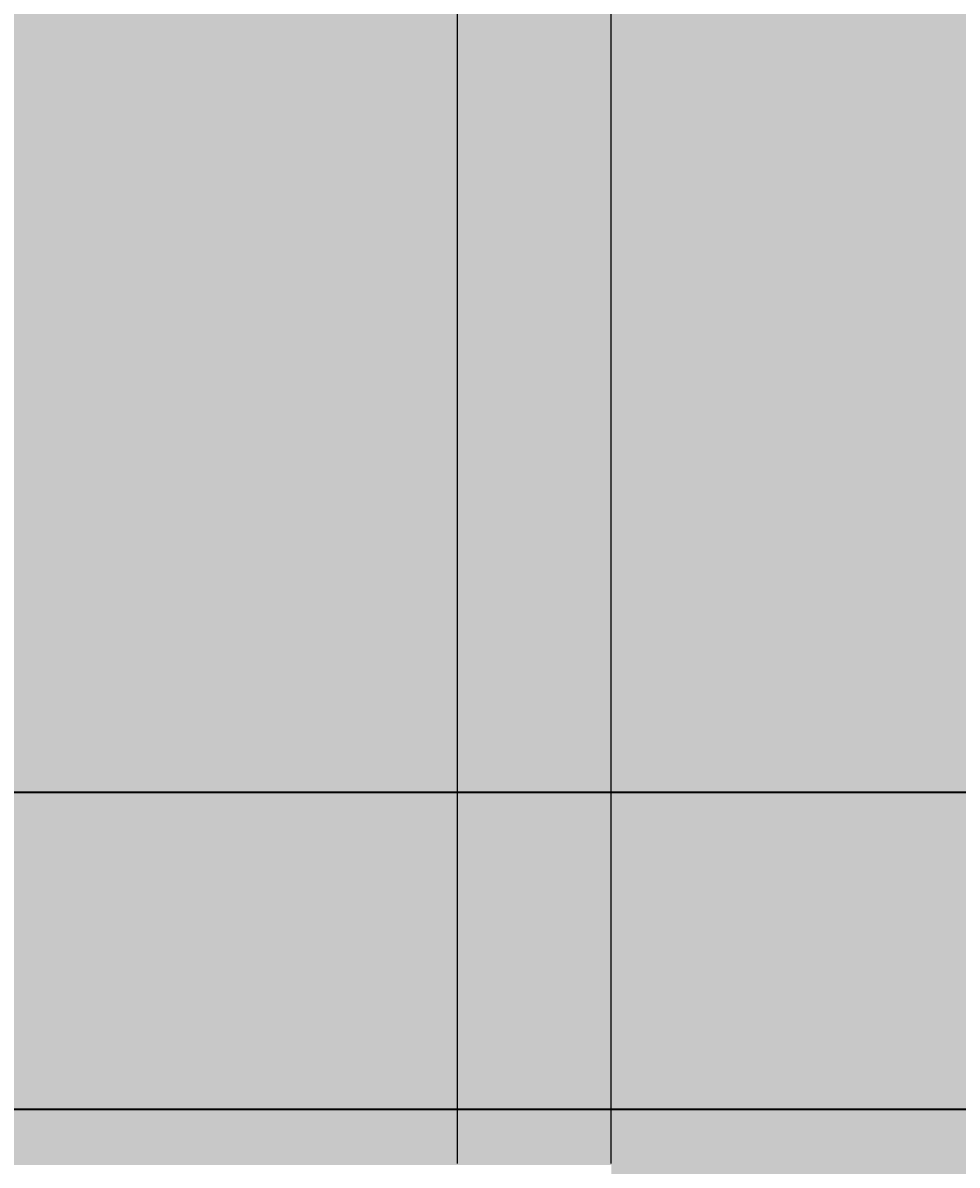
# Model space of a CAD drawing. Units: feet. Extents: x 2695 to 2912, y 795 to 1139.
# Tile 47 of 83: x 2732 to 2769, y 1048 to 1093. Entities that reach past the tile are written whole.
import ezdxf

# ---------------------------------------------------------------- set-up
doc = ezdxf.new("R2010")
doc.units = ezdxf.units.FT
for name, color, linetype, lineweight in [('A-ANNO-DIMS', 2, 'Continuous', 18), ('A-ELEV', 7, 'Continuous', 35), ('A-ELEV-PATT', 252, 'Continuous', 13)]:
    doc.layers.add(name, color=color, linetype=linetype, lineweight=lineweight)
doc.styles.get("Standard").update_dxf_attribs({"font": 'arial.ttf'})
doc.dimstyles.get("Standard").update_dxf_attribs({"dimtxt": 0.18, "dimasz": 0.18, "dimexe": 0.18, "dimexo": 0.0625, "dimgap": 0.09, "dimtad": 0, "dimtih": 1, "dimtoh": 1, "dimdec": 1, "dimzin": 0, "dimdsep": 46, "dimlunit": 3, "dimtxsty": 'Standard', "dimcen": 0.09, "dimadec": 0, "dimazin": 0, "dimtfac": 1, "dimtdec": 1, "dimtofl": 0, "dimtmove": 0, "dimatfit": 3, "dimfxl": 1, "dimtolj": 1, "dimtzin": 0, "dimarcsym": 0})

# ---------------------------------------------------------------- blocks, each defined once
blk = doc.blocks.new('*D8')
at = {"layer": 'A-ANNO-DIMS', "color": 0, "lineweight": -2, "transparency": 16777216}
for p, q in [((2715.885, 1050.373), (2715.885, 1138.886)), ((2770.636, 1122.993), (2770.636, 1138.886)), ((2716.065, 1138.706), (2742.866, 1138.706)), ((2770.456, 1138.706), (2743.655, 1138.706))]:
    blk.add_line(p, q, dxfattribs=at)
at = {"layer": 'A-ANNO-DIMS', "color": 0, "transparency": 16777216}
for points in [[(2716.065, 1138.736), (2716.065, 1138.676), (2715.885, 1138.706)], [(2770.456, 1138.736), (2770.456, 1138.676), (2770.636, 1138.706)]]:
    blk.add_solid(points, dxfattribs=at)
at = {"layer": 'Defpoints', "color": 0, "transparency": 16777216}
for p in [(2770.636, 1138.706), (2770.636, 1122.931), (2715.885, 1050.311)]:
    blk.add_point(p, dxfattribs=at)
at = {"layer": 'A-ANNO-DIMS', "color": 0, "transparency": 16777216, "insert": (2743.261, 1138.706), "char_height": 0.18, "attachment_point": 5}
blk.add_mtext('\\A1;54.75', dxfattribs=at)
blk = doc.blocks.new('*D26')
at = {"layer": 'A-ANNO-DIMS', "color": 0, "lineweight": -2, "transparency": 16777216}
for p, q in [((2749.011, 1048.168), (2749.011, 1138.886)), ((2755.112, 1048.168), (2755.112, 1138.886)), ((2749.191, 1138.706), (2751.685, 1138.706)), ((2754.932, 1138.706), (2752.439, 1138.706))]:
    blk.add_line(p, q, dxfattribs=at)
at = {"layer": 'A-ANNO-DIMS', "color": 0, "transparency": 16777216}
for points in [[(2749.191, 1138.736), (2749.191, 1138.676), (2749.011, 1138.706)], [(2754.932, 1138.736), (2754.932, 1138.676), (2755.112, 1138.706)]]:
    blk.add_solid(points, dxfattribs=at)
at = {"layer": 'Defpoints', "color": 0, "transparency": 16777216}
for p in [(2755.112, 1138.706), (2749.011, 1048.105), (2755.112, 1048.105)]:
    blk.add_point(p, dxfattribs=at)
at = {"layer": 'A-ANNO-DIMS', "color": 0, "transparency": 16777216, "insert": (2752.062, 1138.706), "char_height": 0.18, "attachment_point": 5}
blk.add_mtext('\\A1;6.101', dxfattribs=at)

msp = doc.modelspace()

# ---------------------------------------------------------------- hatches: boundary and pattern name
at = {"layer": 'A-ELEV-PATT'}
h = msp.add_hatch(color=256, dxfattribs=at)
h.set_gradient(color1=(255, 255, 255), tint=1)
h.paths.add_polyline_path([(2770.6361, 1122.9306), (2710.6361, 1122.9306), (2710.6361, 1118.4096), (2770.6361, 1118.4096)])
h.paths.add_polyline_path([(2890.6361, 1107.8588), (2770.6361, 1107.8588), (2770.6361, 1103.3378), (2890.6361, 1103.3378)])
h.paths.add_polyline_path([(2890.6361, 1062.9306), (2710.6361, 1062.9306), (2710.6361, 1056.9306), (2710.6361, 936.9306), (2710.6361, 924.3105), (2716.5358, 924.3105), (2890.6361, 924.3105), (2890.6361, 936.9306), (2715.8852, 936.9306), (2715.8852, 1050.3105), (2890.6361, 1050.3105)])
h.paths.add_polyline_path([(2716.5358, 924.3105), (2710.6361, 924.3105), (2710.6361, 810.9306), (2716.5358, 810.9306)])
h = msp.add_hatch(color=256, dxfattribs=at)
h.set_gradient(color1=(147, 149, 152), color2=(147, 149, 152), tint=1)
h.paths.add_polyline_path([(2770.6361, 1118.4096), (2710.6361, 1118.4096), (2710.6361, 1062.9306), (2770.6361, 1062.9306)])
h.paths.add_polyline_path([(2890.6361, 1103.3378), (2770.6361, 1103.3378), (2770.6361, 1062.9306), (2890.6361, 1062.9306)])
h.paths.add_polyline_path([(2730.7081, 1048.1052), (2755.1125, 1048.1052), (2755.1125, 936.9306), (2770.6361, 936.9306), (2770.6361, 1050.3105), (2715.8852, 1050.3105), (2715.8852, 936.9306), (2730.7081, 936.9306)])
h.paths.add_polyline_path([(2890.6361, 1050.3105), (2770.6361, 1050.3105), (2770.6361, 971.9673), (2778.0341, 971.9673), (2778.0341, 1020.8235), (2843.575, 1020.8235), (2843.575, 971.9673), (2890.6361, 971.9673)])
h.paths.add_polyline_path([(2888.1882, 970.7156), (2843.575, 970.7156), (2843.575, 964.8267), (2888.1882, 964.8267)])
h.paths.add_polyline_path([(2888.1882, 964.1328), (2843.575, 964.1328), (2843.575, 956.614), (2888.1882, 956.614)])
h.paths.add_polyline_path([(2888.1882, 955.9202), (2843.575, 955.9202), (2843.575, 949.2892), (2888.1882, 949.2892)])
h.paths.add_polyline_path([(2888.1882, 948.5954), (2843.575, 948.5954), (2843.575, 941.3507), (2888.1882, 941.3507)])
h.paths.add_polyline_path([(2888.1882, 940.6569), (2843.575, 940.6569), (2843.575, 936.9306), (2888.1882, 936.9306)])
h.paths.add_polyline_path([(2890.6361, 970.7156), (2888.9368, 970.7156), (2888.9368, 964.8267), (2890.6361, 964.8267)])
h.paths.add_polyline_path([(2890.6361, 964.1328), (2888.9368, 964.1328), (2888.9368, 956.614), (2890.6361, 956.614)])
h.paths.add_polyline_path([(2890.6361, 955.9202), (2888.9368, 955.9202), (2888.9368, 949.2892), (2890.6361, 949.2892)])
h.paths.add_polyline_path([(2890.6361, 940.6569), (2888.9368, 940.6569), (2888.9368, 936.9306), (2890.6361, 936.9306)])
h.paths.add_polyline_path([(2890.6361, 948.5954), (2888.9368, 948.5954), (2888.9368, 941.3507), (2890.6361, 941.3507)])
h.paths.add_polyline_path([(2772.5216, 970.7156), (2770.6361, 970.7156), (2770.6361, 964.8267), (2772.5216, 964.8267)])
h.paths.add_polyline_path([(2772.5216, 964.1328), (2770.6361, 964.1328), (2770.6361, 956.614), (2772.5216, 956.614)])
h.paths.add_polyline_path([(2772.5216, 955.9202), (2770.6361, 955.9202), (2770.6361, 949.2892), (2772.5216, 949.2892)])
h.paths.add_polyline_path([(2772.5216, 948.5954), (2770.6361, 948.5954), (2770.6361, 941.3507), (2772.5216, 941.3507)])
h.paths.add_polyline_path([(2772.5216, 940.6569), (2770.6361, 940.6569), (2770.6361, 936.9306), (2772.5216, 936.9306)])
h.paths.add_polyline_path([(2778.0341, 940.6569), (2773.2702, 940.6569), (2773.2702, 936.9306), (2778.0341, 936.9306)])
h.paths.add_polyline_path([(2778.0341, 970.7156), (2773.2702, 970.7156), (2773.2702, 964.8267), (2778.0341, 964.8267)])
h.paths.add_polyline_path([(2778.0341, 964.1328), (2773.2702, 964.1328), (2773.2702, 956.614), (2778.0341, 956.614)])
h.paths.add_polyline_path([(2778.0341, 955.9202), (2773.2702, 955.9202), (2773.2702, 949.2892), (2778.0341, 949.2892)])
h.paths.add_polyline_path([(2778.0341, 948.5954), (2773.2702, 948.5954), (2773.2702, 941.3507), (2778.0341, 941.3507)])
h.paths.add_polyline_path([(2810.0407, 940.6569), (2780.0341, 940.6569), (2780.0341, 936.9306), (2810.0407, 936.9306)])
h.paths.add_polyline_path([(2890.6361, 924.3105), (2770.6361, 924.3105), (2770.6361, 810.9306), (2773.5029, 810.9306), (2773.5029, 905.5143), (2805.9398, 905.5143), (2838.3767, 905.5143), (2838.3767, 810.9306), (2890.6361, 810.9306)])

# ---------------------------------------------------------------- linework, layer by layer
at = {"layer": 'A-ELEV'}
for p, q in [((2710.6361, 1062.9306), (2890.6361, 1062.9306)), ((2710.6361, 1062.9306), (2895.4694, 1062.9306)), ((2890.6361, 1050.3105), (2715.8852, 1050.3105))]:
    msp.add_line(p, q, dxfattribs=at)
msp.add_lwpolyline([(2890.6361, 1050.3105), (2715.8852, 1050.3105)], dxfattribs=at)

# ---------------------------------------------------------------- dimensions: what is measured, and where the dimension line sits
at = {"layer": 'A-ANNO-DIMS'}
for base, p1, p2, override, picture, middle in [((2770.6361, 1138.7056), (2715.8852, 1050.3105), (2770.6361, 1122.9306), {"dimdec": 2, "dimlfac": 1, "dimrnd": 0, "dimzin": 0, "dimdsep": 46, "dimlunit": 2}, '*D8', (2743.2606, 1138.7056)), ((2755.1125, 1138.7056), (2749.0114, 1048.1052), (2755.1125, 1048.1052), {"dimdec": 3, "dimlfac": 1, "dimrnd": 0, "dimzin": 0, "dimdsep": 46, "dimlunit": 2}, '*D26', (2752.0619, 1138.7056))]:
    dim = msp.add_linear_dim(base=base, p1=p1, p2=p2, dimstyle='Standard', override=override, dxfattribs=at)
    dim.commit()
    dim.dimension.update_dxf_attribs({"geometry": picture, "text_midpoint": middle})

doc.saveas('drawing.dxf')
